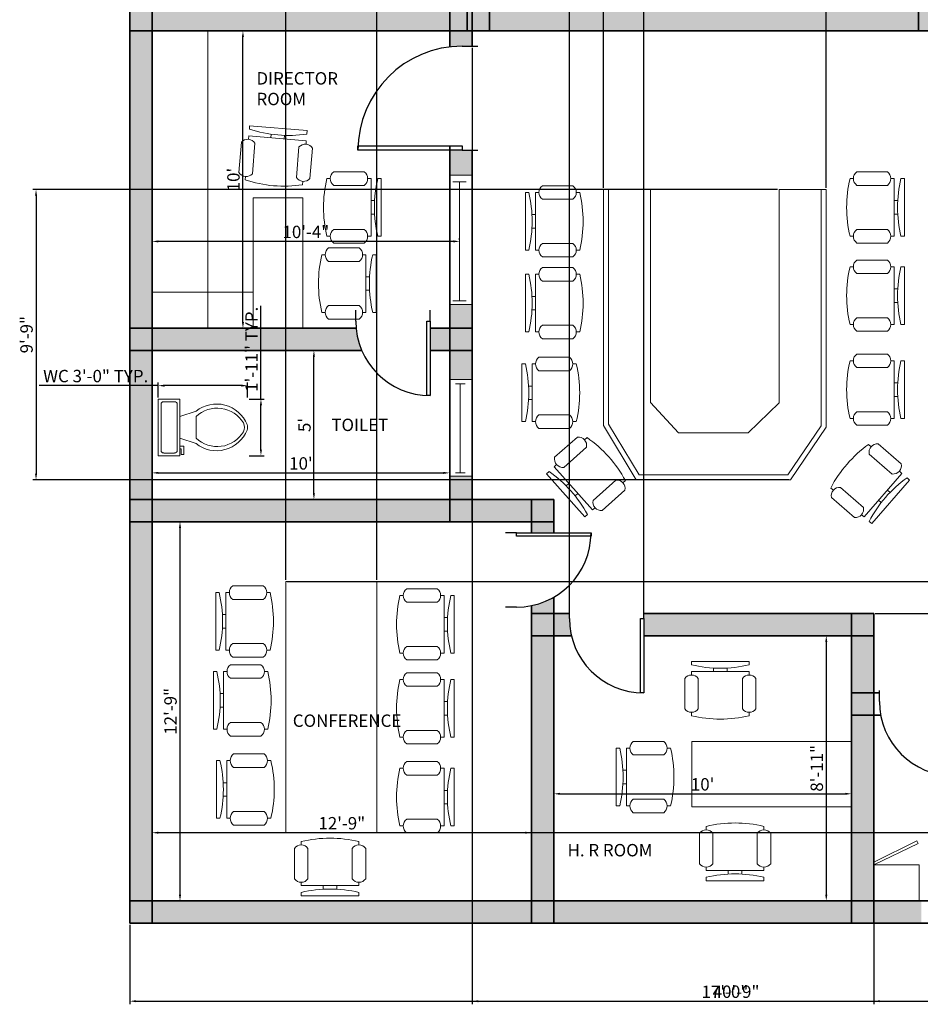
# Model space of a CAD drawing. Units: millimetres. Extents: x 2436 to 3005, y 774 to 1472.
# Tile 1 of 3: x 2436 to 2799, y 774 to 1172. Entities that reach past the tile are written whole.
import ezdxf

# ---------------------------------------------------------------- set-up
doc = ezdxf.new("R2010")
doc.units = ezdxf.units.MM
for name, color, linetype, lineweight in [('A-ANNO-DIMS', 2, 'Continuous', 18), ('A-AREA-IDEN', 10, 'Continuous', 25), ('A-FLOR-CASE', 140, 'Continuous', 18), ('A-FLOR-FIXT', 140, 'Continuous', 18), ('A-WALL-PATT', 3, 'Continuous', 13), ('doors', 30, 'Continuous', 25), ('furniture', 140, 'Continuous', 18), ('walls', 80, 'Continuous', 35), ('window', 190, 'Continuous', 20)]:
    doc.layers.add(name, color=color, linetype=linetype, lineweight=lineweight)
doc.styles.get("Standard").update_dxf_attribs({"font": 'arial.ttf'})
doc.dimstyles.new('ISO-25', dxfattribs={"dimtxt": 5, "dimasz": 2.5, "dimexe": 1.25, "dimexo": 0.625, "dimtad": 1, "dimdec": 0, "dimlunit": 3, "dimtxsty": 'Standard', "dimcen": 2.5, "dimadec": 0, "dimazin": 0, "dimtfac": 1, "dimtdec": 0, "dimtmove": 0, "dimatfit": 3, "dimfxl": 1, "dimarcsym": 0})

# ---------------------------------------------------------------- blocks, each defined once
blk = doc.blocks.new('*U2')
for p, q in [((0, 0), (0, -6)), ((40, 0), (40, -6))]:
    blk.add_line(p, q)
blk.add_lwpolyline([(0, 0), (0, 40), (1.75, 40), (1.75, 0)], close=True)
blk.add_arc((0, 0), 40, 0, 90)
blk = doc.blocks.new('*U4')
for p, q in [((0, 4), (0, 0)), ((36, 4), (36, 0)), ((0, 2), (36, 2))]:
    blk.add_line(p, q)
blk = doc.blocks.new('*U5')
for p, q in [((0, 4), (0, 0)), ((36, 4), (36, 0)), ((0, 2), (36, 2))]:
    blk.add_line(p, q)
blk = doc.blocks.new('Chair - Desk')
for p, q in [((-8.5, 0), (-8.5, -1)), ((-8.5, 0), (8.5, 0)), ((8.5, 0), (8.5, -1)), ((-2, -3), (-2, -1.9355)), ((2, -1.9576), (2, -3)), ((-10.5, -5), (-10.5, -14)), ((-8.5, -3), (-8.5, -4)), ((-8.5, -3), (8.5, -3)), ((-6.5, -14), (-6.5, -5)), ((6.5, -5), (6.5, -14)), ((8.5, -3), (8.5, -4)), ((10.5, -14), (10.5, -5)), ((-8.5, -15), (-8.5, -16)), ((8.5, -15), (8.5, -16))]:
    blk.add_line(p, q)
for centre, radius, start, end in [((0, 34.625), 36.625, 256.5803, 283.4197), ((-8.5, -6.5), 2.5, 36.8699, 143.1301), ((8.5, -6.5), 2.5, 36.8699, 143.1301), ((-8.5, -12.5), 2.5, 216.8699, 323.1301), ((8.5, -12.5), 2.5, 216.8699, 323.1301), ((0, 19.625), 36.625, 256.5803, 283.4197)]:
    blk.add_arc(centre, radius, start, end)
blk = doc.blocks.new('Toilet - top')
for p, q in [((9.5, -6), (9.5, -2)), ((-10, -8.5), (-8, -8.5)), ((-10, -9.5), (-10, -8.5)), ((-7, -9.5), (-10, -9.5)), ((-8, -8.5), (-8, -8)), ((-7, -8), (-7, -9.5)), ((-4, -8), (-6, -14)), ((4, -8), (6, -14)), ((4, -14), (-4, -14))]:
    blk.add_line(p, q)
blk.add_lwpolyline([(10.5, -8), (10.5, 0), (-10.5, 0), (-10.5, -8)], close=True)
for points in [[(-9.5, -2), (-9.5, -6)], [(8.5, -1), (-8.5, -1)], [(-8.5, -7), (8.5, -7)]]:
    blk.add_lwpolyline(points)
for centre, radius, start, end in [((-8.62, -1.88), 0.884, 81.8699, 188.1301), ((8.62, -1.88), 0.884, 351.8699, 98.1301), ((-8.62, -6.12), 0.884, 171.8699, 278.1301), ((8.62, -6.12), 0.884, 261.8699, 8.1301), ((3.52, -21.58), 12.17, 141.4691, 247.9714), ((4.2, -21.82), 11.33, 136.3677, 238.9468), ((-3.52, -21.58), 12.17, 292.0284, 38.5307), ((-4.2, -21.82), 11.33, 301.053, 43.6321), ((0, -27.88), 4, 245.7318, 294.2682), ((0, -29), 4, 254.8605, 285.1395)]:
    blk.add_arc(centre, radius, start, end)
blk = doc.blocks.new('*D17')
at = {"layer": 'A-ANNO-DIMS', "color": 0, "lineweight": -2, "transparency": 16777216}
for p, q in [((2525.92, 1049.62), (2525.92, 1164.62)), ((2526.54, 1167.12), (2527.17, 1167.12)), ((2526.54, 1047.12), (2527.17, 1047.12))]:
    blk.add_line(p, q, dxfattribs=at)
at = {"layer": 'A-ANNO-DIMS', "color": 0, "transparency": 16777216}
for points in [[(2525.5, 1164.62), (2526.33, 1164.62), (2525.92, 1167.12)], [(2525.5, 1049.62), (2526.33, 1049.62), (2525.92, 1047.12)]]:
    blk.add_solid(points, dxfattribs=at)
at = {"layer": 'Defpoints', "color": 0, "transparency": 16777216}
for p in [(2525.92, 1167.12), (2525.92, 1167.12), (2525.92, 1047.12)]:
    blk.add_point(p, dxfattribs=at)
at = {"layer": 'A-ANNO-DIMS', "color": 0, "transparency": 16777216, "insert": (2522.74, 1107.12), "char_height": 5, "attachment_point": 5, "rotation": 90}
blk.add_mtext("10'", dxfattribs=at)
blk = doc.blocks.new('*D18')
at = {"layer": 'A-ANNO-DIMS', "color": 0, "lineweight": -2, "transparency": 16777216}
for p, q in [((2489.3, 1082.81), (2489.3, 1083.44)), ((2610.8, 1082.19), (2491.8, 1082.19)), ((2613.3, 1082.81), (2613.3, 1083.44))]:
    blk.add_line(p, q, dxfattribs=at)
at = {"layer": 'A-ANNO-DIMS', "color": 0, "transparency": 16777216}
for points in [[(2491.8, 1082.6), (2491.8, 1081.77), (2489.3, 1082.19)], [(2610.8, 1082.6), (2610.8, 1081.77), (2613.3, 1082.19)]]:
    blk.add_solid(points, dxfattribs=at)
at = {"layer": 'Defpoints', "color": 0, "transparency": 16777216}
for p in [(2489.3, 1082.19), (2489.3, 1082.19), (2613.3, 1082.19)]:
    blk.add_point(p, dxfattribs=at)
at = {"layer": 'A-ANNO-DIMS', "color": 0, "transparency": 16777216, "insert": (2551.3, 1085.36), "char_height": 5, "attachment_point": 5}
blk.add_mtext('10\'-4"', dxfattribs=at)
blk = doc.blocks.new('*D19')
at = {"layer": 'A-ANNO-DIMS', "color": 0, "lineweight": -2, "transparency": 16777216}
for p, q in [((2553.44, 1038.12), (2555.79, 1038.12)), ((2554.54, 980.62), (2554.54, 1035.62)), ((2553.44, 978.12), (2555.79, 978.12))]:
    blk.add_line(p, q, dxfattribs=at)
at = {"layer": 'A-ANNO-DIMS', "color": 0, "transparency": 16777216}
for points in [[(2554.12, 1035.62), (2554.96, 1035.62), (2554.54, 1038.12)], [(2554.12, 980.62), (2554.96, 980.62), (2554.54, 978.12)]]:
    blk.add_solid(points, dxfattribs=at)
at = {"layer": 'Defpoints', "color": 0, "transparency": 16777216}
for p in [(2552.81, 1038.12), (2554.54, 1038.12), (2552.81, 978.12)]:
    blk.add_point(p, dxfattribs=at)
at = {"layer": 'A-ANNO-DIMS', "color": 0, "transparency": 16777216, "insert": (2551.37, 1008.12), "char_height": 5, "attachment_point": 5, "rotation": 90}
blk.add_mtext("5'", dxfattribs=at)
blk = doc.blocks.new('*D20')
at = {"layer": 'A-ANNO-DIMS', "color": 0, "lineweight": -2, "transparency": 16777216}
for p, q in [((2489.3, 987.7), (2489.3, 990.05)), ((2609.3, 987.7), (2609.3, 990.05)), ((2491.8, 988.8), (2606.8, 988.8))]:
    blk.add_line(p, q, dxfattribs=at)
at = {"layer": 'A-ANNO-DIMS', "color": 0, "transparency": 16777216}
for points in [[(2491.8, 989.22), (2491.8, 988.39), (2489.3, 988.8)], [(2606.8, 989.22), (2606.8, 988.39), (2609.3, 988.8)]]:
    blk.add_solid(points, dxfattribs=at)
at = {"layer": 'Defpoints', "color": 0, "transparency": 16777216}
for p in [(2489.3, 987.08), (2609.3, 988.8), (2609.3, 987.08)]:
    blk.add_point(p, dxfattribs=at)
at = {"layer": 'A-ANNO-DIMS', "color": 0, "transparency": 16777216, "insert": (2549.3, 991.98), "char_height": 5, "attachment_point": 5}
blk.add_mtext("10'", dxfattribs=at)
blk = doc.blocks.new('*D21')
at = {"layer": 'A-ANNO-DIMS', "color": 0, "lineweight": -2, "transparency": 16777216}
for p, q in [((2494.98, 969.12), (2501.78, 969.12)), ((2500.53, 966.62), (2500.53, 818.62)), ((2494.98, 816.12), (2501.78, 816.12))]:
    blk.add_line(p, q, dxfattribs=at)
at = {"layer": 'A-ANNO-DIMS', "color": 0, "transparency": 16777216}
for points in [[(2500.12, 966.62), (2500.95, 966.62), (2500.53, 969.12)], [(2500.12, 818.62), (2500.95, 818.62), (2500.53, 816.12)]]:
    blk.add_solid(points, dxfattribs=at)
at = {"layer": 'Defpoints', "color": 0, "transparency": 16777216}
for p in [(2494.35, 969.12), (2494.35, 816.12), (2500.53, 816.12)]:
    blk.add_point(p, dxfattribs=at)
at = {"layer": 'A-ANNO-DIMS', "color": 0, "transparency": 16777216, "insert": (2497.36, 892.62), "char_height": 5, "attachment_point": 5, "rotation": 90}
blk.add_mtext('12\'-9"', dxfattribs=at)
blk = doc.blocks.new('*D22')
at = {"layer": 'A-ANNO-DIMS', "color": 0, "lineweight": -2, "transparency": 16777216}
for p, q in [((2489.3, 844.27), (2489.3, 844.89)), ((2639.8, 843.64), (2491.8, 843.64)), ((2642.3, 844.27), (2642.3, 844.89))]:
    blk.add_line(p, q, dxfattribs=at)
at = {"layer": 'A-ANNO-DIMS', "color": 0, "transparency": 16777216}
for points in [[(2491.8, 844.06), (2491.8, 843.23), (2489.3, 843.64)], [(2639.8, 844.06), (2639.8, 843.23), (2642.3, 843.64)]]:
    blk.add_solid(points, dxfattribs=at)
at = {"layer": 'Defpoints', "color": 0, "transparency": 16777216}
for p in [(2489.3, 843.64), (2489.3, 843.64), (2642.3, 843.64)]:
    blk.add_point(p, dxfattribs=at)
at = {"layer": 'A-ANNO-DIMS', "color": 0, "transparency": 16777216, "insert": (2565.8, 846.82), "char_height": 5, "attachment_point": 5}
blk.add_mtext('12\'-9"', dxfattribs=at)
blk = doc.blocks.new('*D23')
at = {"layer": 'A-ANNO-DIMS', "color": 0, "lineweight": -2, "transparency": 16777216}
for p, q in [((2651.3, 865.17), (2651.3, 858.09)), ((2771.3, 865.17), (2771.3, 858.09)), ((2653.8, 859.34), (2768.8, 859.34))]:
    blk.add_line(p, q, dxfattribs=at)
at = {"layer": 'A-ANNO-DIMS', "color": 0, "transparency": 16777216}
for points in [[(2653.8, 859.76), (2653.8, 858.92), (2651.3, 859.34)], [(2768.8, 859.76), (2768.8, 858.92), (2771.3, 859.34)]]:
    blk.add_solid(points, dxfattribs=at)
at = {"layer": 'Defpoints', "color": 0, "transparency": 16777216}
for p in [(2651.3, 865.79), (2771.3, 865.79), (2771.3, 859.34)]:
    blk.add_point(p, dxfattribs=at)
at = {"layer": 'A-ANNO-DIMS', "color": 0, "transparency": 16777216, "insert": (2711.3, 862.52), "char_height": 5, "attachment_point": 5}
blk.add_mtext("10'", dxfattribs=at)
blk = doc.blocks.new('*D24')
at = {"layer": 'A-ANNO-DIMS', "color": 0, "lineweight": -2, "transparency": 16777216}
for p, q in [((2758.99, 923.12), (2762.41, 923.12)), ((2761.16, 920.62), (2761.16, 818.62)), ((2761.79, 816.12), (2762.41, 816.12))]:
    blk.add_line(p, q, dxfattribs=at)
at = {"layer": 'A-ANNO-DIMS', "color": 0, "transparency": 16777216}
for points in [[(2760.75, 920.62), (2761.58, 920.62), (2761.16, 923.12)], [(2760.75, 818.62), (2761.58, 818.62), (2761.16, 816.12)]]:
    blk.add_solid(points, dxfattribs=at)
at = {"layer": 'Defpoints', "color": 0, "transparency": 16777216}
for p in [(2758.36, 923.12), (2761.16, 816.12), (2761.16, 816.12)]:
    blk.add_point(p, dxfattribs=at)
at = {"layer": 'A-ANNO-DIMS', "color": 0, "transparency": 16777216, "insert": (2757.99, 869.62), "char_height": 5, "attachment_point": 5, "rotation": 90}
blk.add_mtext('8\'-11"', dxfattribs=at)
blk = doc.blocks.new('*D36')
at = {"layer": 'A-ANNO-DIMS', "color": 0, "lineweight": -2, "transparency": 16777216}
for p, q in [((2491.79, 1019.23), (2491.79, 1025.25)), ((2527.78, 1019.23), (2527.78, 1025.25)), ((2491.79, 1024), (2443.78, 1024)), ((2525.28, 1024), (2494.29, 1024))]:
    blk.add_line(p, q, dxfattribs=at)
at = {"layer": 'A-ANNO-DIMS', "color": 0, "transparency": 16777216}
for points in [[(2494.29, 1024.42), (2494.29, 1023.58), (2491.79, 1024)], [(2525.28, 1024.42), (2525.28, 1023.58), (2527.78, 1024)]]:
    blk.add_solid(points, dxfattribs=at)
at = {"layer": 'Defpoints', "color": 0, "transparency": 16777216}
for p in [(2491.79, 1024), (2491.79, 1018.6), (2527.78, 1018.6)]:
    blk.add_point(p, dxfattribs=at)
at = {"layer": 'A-ANNO-DIMS', "color": 0, "transparency": 16777216, "insert": (2466.54, 1027.21), "char_height": 5, "attachment_point": 5}
blk.add_mtext('WC 3\'-0" TYP.', dxfattribs=at)
blk = doc.blocks.new('*D37')
at = {"layer": 'A-ANNO-DIMS', "color": 0, "lineweight": -2, "transparency": 16777216}
for p, q in [((2533.18, 1018.6), (2533.18, 1056.24)), ((2528.41, 1018.6), (2534.43, 1018.6)), ((2533.18, 998.23), (2533.18, 1016.1)), ((2528.41, 995.73), (2534.43, 995.73))]:
    blk.add_line(p, q, dxfattribs=at)
at = {"layer": 'A-ANNO-DIMS', "color": 0, "transparency": 16777216}
for points in [[(2532.76, 1016.1), (2533.6, 1016.1), (2533.18, 1018.6)], [(2532.76, 998.23), (2533.6, 998.23), (2533.18, 995.73)]]:
    blk.add_solid(points, dxfattribs=at)
at = {"layer": 'Defpoints', "color": 0, "transparency": 16777216}
for p in [(2527.78, 1018.6), (2533.18, 1018.6), (2527.78, 995.73)]:
    blk.add_point(p, dxfattribs=at)
at = {"layer": 'A-ANNO-DIMS', "color": 0, "transparency": 16777216, "insert": (2530.04, 1038.67), "char_height": 5, "attachment_point": 5, "rotation": 90}
blk.add_mtext('1\'-11" TYP.', dxfattribs=at)
blk = doc.blocks.new('*D40')
at = {"layer": 'A-ANNO-DIMS', "color": 0, "lineweight": -2, "transparency": 16777216}
for p, q in [((2480.3, 806.5), (2480.3, 774.42)), ((2969.3, 806.5), (2969.3, 774.42)), ((2482.8, 775.67), (2966.8, 775.67))]:
    blk.add_line(p, q, dxfattribs=at)
at = {"layer": 'A-ANNO-DIMS', "color": 0, "transparency": 16777216}
for points in [[(2482.8, 776.09), (2482.8, 775.26), (2480.3, 775.67)], [(2966.8, 776.09), (2966.8, 775.26), (2969.3, 775.67)]]:
    blk.add_solid(points, dxfattribs=at)
at = {"layer": 'Defpoints', "color": 0, "transparency": 16777216}
for p in [(2480.3, 807.12), (2969.3, 807.12), (2969.3, 775.67)]:
    blk.add_point(p, dxfattribs=at)
at = {"layer": 'A-ANNO-DIMS', "color": 0, "transparency": 16777216, "insert": (2724.8, 778.85), "char_height": 5, "attachment_point": 5}
blk.add_mtext('40\'-9"', dxfattribs=at)
blk = doc.blocks.new('*D42')
at = {"layer": 'A-ANNO-DIMS', "color": 0, "lineweight": -2, "transparency": 16777216}
for p, q in [((2780.3, 931.5), (2780.3, 774.42)), ((2960.3, 890.5), (2960.3, 774.42)), ((2782.8, 775.67), (2957.8, 775.67))]:
    blk.add_line(p, q, dxfattribs=at)
at = {"layer": 'A-ANNO-DIMS', "color": 0, "transparency": 16777216}
for points in [[(2782.8, 776.09), (2782.8, 775.26), (2780.3, 775.67)], [(2957.8, 776.09), (2957.8, 775.26), (2960.3, 775.67)]]:
    blk.add_solid(points, dxfattribs=at)
at = {"layer": 'Defpoints', "color": 0, "transparency": 16777216}
for p in [(2780.3, 932.12), (2960.3, 891.12), (2960.3, 775.67)]:
    blk.add_point(p, dxfattribs=at)
at = {"layer": 'A-ANNO-DIMS', "color": 0, "transparency": 16777216, "insert": (2870.3, 778.85), "char_height": 5, "attachment_point": 5}
blk.add_mtext('15\'-0"', dxfattribs=at)
blk = doc.blocks.new('*D43')
at = {"layer": 'A-ANNO-DIMS', "color": 0, "lineweight": -2, "transparency": 16777216}
for p, q in [((2822.3, 1175.5), (2822.3, 774.42)), ((2618.3, 1160.31), (2618.3, 774.42)), ((2620.8, 775.67), (2819.8, 775.67))]:
    blk.add_line(p, q, dxfattribs=at)
at = {"layer": 'A-ANNO-DIMS', "color": 0, "transparency": 16777216}
for points in [[(2620.8, 776.09), (2620.8, 775.26), (2618.3, 775.67)], [(2819.8, 776.09), (2819.8, 775.26), (2822.3, 775.67)]]:
    blk.add_solid(points, dxfattribs=at)
at = {"layer": 'Defpoints', "color": 0, "transparency": 16777216}
for p in [(2822.3, 1176.12), (2618.3, 1160.93), (2822.3, 775.67)]:
    blk.add_point(p, dxfattribs=at)
at = {"layer": 'A-ANNO-DIMS', "color": 0, "transparency": 16777216, "insert": (2720.3, 778.85), "char_height": 5, "attachment_point": 5}
blk.add_mtext('17\'-0"', dxfattribs=at)
blk = doc.blocks.new('*D44')
at = {"layer": 'A-ANNO-DIMS', "color": 0, "lineweight": -2, "transparency": 16777216}
for p, q in [((2798.92, 1167.12), (3002, 1167.12)), ((3000.75, 1164.62), (3000.75, 934.62)), ((2780.92, 932.12), (3002, 932.12))]:
    blk.add_line(p, q, dxfattribs=at)
at = {"layer": 'A-ANNO-DIMS', "color": 0, "transparency": 16777216}
for points in [[(3000.33, 1164.62), (3001.17, 1164.62), (3000.75, 1167.12)], [(3000.33, 934.62), (3001.17, 934.62), (3000.75, 932.12)]]:
    blk.add_solid(points, dxfattribs=at)
at = {"layer": 'Defpoints', "color": 0, "transparency": 16777216}
for p in [(2798.3, 1167.12), (2780.3, 932.12), (3000.75, 932.12)]:
    blk.add_point(p, dxfattribs=at)
at = {"layer": 'A-ANNO-DIMS', "color": 0, "transparency": 16777216, "insert": (2997.57, 1049.62), "char_height": 5, "attachment_point": 5, "rotation": 90}
blk.add_mtext('19\'-7"', dxfattribs=at)
blk = doc.blocks.new('*D49')
at = {"layer": 'A-ANNO-DIMS', "color": 0, "lineweight": -2, "transparency": 16777216}
for p, q in [((2671.31, 1103.79), (2671.31, 1466.82)), ((2761.12, 1103.79), (2761.12, 1466.82)), ((2673.81, 1465.57), (2758.62, 1465.57))]:
    blk.add_line(p, q, dxfattribs=at)
at = {"layer": 'A-ANNO-DIMS', "color": 0, "transparency": 16777216}
for points in [[(2673.81, 1465.99), (2673.81, 1465.16), (2671.31, 1465.57)], [(2758.62, 1465.99), (2758.62, 1465.16), (2761.12, 1465.57)]]:
    blk.add_solid(points, dxfattribs=at)
at = {"layer": 'Defpoints', "color": 0, "transparency": 16777216}
for p in [(2761.12, 1465.57), (2671.31, 1103.17), (2761.12, 1103.17)]:
    blk.add_point(p, dxfattribs=at)
at = {"layer": 'A-ANNO-DIMS', "color": 0, "transparency": 16777216, "insert": (2716.21, 1468.75), "char_height": 5, "attachment_point": 5}
blk.add_mtext('7\'-6"', dxfattribs=at)
blk = doc.blocks.new('*D50')
at = {"layer": 'A-ANNO-DIMS', "color": 0, "lineweight": -2, "transparency": 16777216}
for p, q in [((2741.49, 1103.17), (2441.22, 1103.17)), ((2442.47, 1100.67), (2442.47, 988.45)), ((2746.13, 985.95), (2441.22, 985.95))]:
    blk.add_line(p, q, dxfattribs=at)
at = {"layer": 'A-ANNO-DIMS', "color": 0, "transparency": 16777216}
for points in [[(2442.06, 1100.67), (2442.89, 1100.67), (2442.47, 1103.17)], [(2442.06, 988.45), (2442.89, 988.45), (2442.47, 985.95)]]:
    blk.add_solid(points, dxfattribs=at)
at = {"layer": 'Defpoints', "color": 0, "transparency": 16777216}
for p in [(2742.12, 1103.17), (2442.47, 985.95), (2746.76, 985.95)]:
    blk.add_point(p, dxfattribs=at)
at = {"layer": 'A-ANNO-DIMS', "color": 0, "transparency": 16777216, "insert": (2439.29, 1044.56), "char_height": 5, "attachment_point": 5, "rotation": 90}
blk.add_mtext('9\'-9"', dxfattribs=at)
blk = doc.blocks.new('*D52')
at = {"layer": 'A-ANNO-DIMS', "color": 0, "lineweight": -2, "transparency": 16777216}
for p, q in [((2657.55, 932.75), (2657.55, 1466.82)), ((2687.55, 932.75), (2687.55, 1466.82)), ((2660.05, 1465.57), (2685.05, 1465.57))]:
    blk.add_line(p, q, dxfattribs=at)
at = {"layer": 'A-ANNO-DIMS', "color": 0, "transparency": 16777216}
for points in [[(2660.05, 1465.99), (2660.05, 1465.16), (2657.55, 1465.57)], [(2685.05, 1465.99), (2685.05, 1465.16), (2687.55, 1465.57)]]:
    blk.add_solid(points, dxfattribs=at)
at = {"layer": 'Defpoints', "color": 0, "transparency": 16777216}
for p in [(2687.55, 1465.57), (2657.55, 932.12), (2687.55, 932.12)]:
    blk.add_point(p, dxfattribs=at)
at = {"layer": 'A-ANNO-DIMS', "color": 0, "transparency": 16777216, "insert": (2672.55, 1468.75), "char_height": 5, "attachment_point": 5}
blk.add_mtext('2\'-6"', dxfattribs=at)
blk = doc.blocks.new('*D53')
at = {"layer": 'A-ANNO-DIMS', "color": 0, "lineweight": -2, "transparency": 16777216}
for p, q in [((2543.16, 945.65), (2543.16, 1466.82)), ((2579.92, 945.65), (2579.92, 1466.82)), ((2545.66, 1465.57), (2577.42, 1465.57))]:
    blk.add_line(p, q, dxfattribs=at)
at = {"layer": 'A-ANNO-DIMS', "color": 0, "transparency": 16777216}
for points in [[(2545.66, 1465.99), (2545.66, 1465.16), (2543.16, 1465.57)], [(2577.42, 1465.99), (2577.42, 1465.16), (2579.92, 1465.57)]]:
    blk.add_solid(points, dxfattribs=at)
at = {"layer": 'Defpoints', "color": 0, "transparency": 16777216}
for p in [(2579.92, 1465.57), (2543.16, 945.02), (2579.92, 945.02)]:
    blk.add_point(p, dxfattribs=at)
at = {"layer": 'A-ANNO-DIMS', "color": 0, "transparency": 16777216, "insert": (2561.54, 1468.75), "char_height": 5, "attachment_point": 5}
blk.add_mtext('3\'-1"', dxfattribs=at)
blk = doc.blocks.new('*D54')
at = {"layer": 'A-ANNO-DIMS', "color": 0, "lineweight": -2, "transparency": 16777216}
for p, q in [((2543.78, 945.02), (3002, 945.02)), ((3000.75, 942.52), (3000.75, 846.17)), ((2543.78, 843.67), (3002, 843.67))]:
    blk.add_line(p, q, dxfattribs=at)
at = {"layer": 'A-ANNO-DIMS', "color": 0, "transparency": 16777216}
for points in [[(3000.33, 942.52), (3001.17, 942.52), (3000.75, 945.02)], [(3000.33, 846.17), (3001.17, 846.17), (3000.75, 843.67)]]:
    blk.add_solid(points, dxfattribs=at)
at = {"layer": 'Defpoints', "color": 0, "transparency": 16777216}
for p in [(2543.16, 945.02), (2543.16, 843.67), (3000.75, 843.67)]:
    blk.add_point(p, dxfattribs=at)
at = {"layer": 'A-ANNO-DIMS', "color": 0, "transparency": 16777216, "insert": (2997.54, 894.35), "char_height": 5, "attachment_point": 5, "rotation": 90}
blk.add_mtext('8\'-5 1/2"', dxfattribs=at)

msp = doc.modelspace()

# ---------------------------------------------------------------- hatches: boundary and pattern name
at = {"layer": 'A-WALL-PATT'}
h = msp.add_hatch(color=256, dxfattribs=at)
h.dxf.hatch_style = 1
h.paths.add_polyline_path([(2822.3, 1374.12), (2489.3, 1374.12), (2489.3, 1365.12), (2822.3, 1365.12)])
h.paths.add_polyline_path([(2831.3, 1374.12), (2822.3, 1374.12), (2822.3, 1365.12), (2831.3, 1365.12)])
h.paths.add_polyline_path([(2831.3, 1365.12), (2822.3, 1365.12), (2822.3, 1353.75), (2824.37, 1353.75, -0.041466), (2831.3, 1353.17)])
h.paths.add_polyline_path([(2960.3, 1425.12), (2951.3, 1425.12), (2951.3, 1305.12), (2960.3, 1305.12)])
h.paths.add_polyline_path([(2960.3, 1434.12), (2951.3, 1434.12), (2951.3, 1425.12), (2960.3, 1425.12)])
h.paths.add_polyline_path([(2951.3, 1434.12), (2831.3, 1434.12), (2831.3, 1425.12), (2951.3, 1425.12)])
h.paths.add_polyline_path([(2831.3, 1434.12), (2822.3, 1434.12), (2822.3, 1425.12), (2831.3, 1425.12)])
h.paths.add_polyline_path([(2489.3, 1374.12), (2480.3, 1374.12), (2480.3, 1365.12), (2489.3, 1365.12)])
h.paths.add_polyline_path([(2489.3, 1365.12), (2480.3, 1365.12), (2480.3, 1354.49), (2489.3, 1354.89)])
h.paths.add_polyline_path([(2489.3, 1313.48, -0.04329), (2482.1, 1312.53), (2480.3, 1312.44), (2480.3, 1176.12), (2489.3, 1176.12)])
h.paths.add_polyline_path([(2489.3, 1176.12), (2480.3, 1176.12), (2480.3, 1167.12), (2489.3, 1167.12)])
h.paths.add_polyline_path([(2609.3, 1176.12), (2489.3, 1176.12), (2489.3, 1167.12), (2609.3, 1167.12)])
h.paths.add_polyline_path([(2625.3, 1176.12), (2618.3, 1176.12), (2618.3, 1167.12), (2625.3, 1167.12)])
h.paths.add_polyline_path([(2618.3, 1176.12), (2616.3, 1176.12), (2616.3, 1167.12), (2618.3, 1167.12)])
h.paths.add_polyline_path([(2616.3, 1176.12), (2609.3, 1176.12), (2609.3, 1167.12), (2616.3, 1167.12)])
h.paths.add_polyline_path([(2618.3, 1167.12), (2609.3, 1167.12), (2609.3, 1160.63, -0.029892), (2614.31, 1160.93), (2618.3, 1160.93)])
h.paths.add_polyline_path([(2625.3, 1305.12), (2616.3, 1305.12), (2616.3, 1176.12), (2618.3, 1176.12), (2625.3, 1176.12)])
h.paths.add_polyline_path([(2798.3, 1176.12), (2625.3, 1176.12), (2625.3, 1167.12), (2798.3, 1167.12)])
h.paths.add_polyline_path([(2807.3, 1176.12), (2798.3, 1176.12), (2798.3, 1167.12), (2807.3, 1167.12)])
h.paths.add_polyline_path([(2831.3, 1176.12), (2822.3, 1176.12), (2822.3, 1167.12), (2831.3, 1167.12)])
h.paths.add_polyline_path([(2822.3, 1176.12), (2807.3, 1176.12), (2807.3, 1167.12), (2822.3, 1167.12)])
h.paths.add_polyline_path([(2951.3, 1176.12), (2831.3, 1176.12), (2831.3, 1167.12), (2951.3, 1167.12)])
h.paths.add_polyline_path([(2960.3, 1176.12), (2951.3, 1176.12), (2951.3, 1167.12), (2960.3, 1167.12)])
h.paths.add_polyline_path([(2960.3, 1296.12), (2951.3, 1296.12), (2951.3, 1176.12), (2960.3, 1176.12)])
h.paths.add_polyline_path([(2960.3, 1305.12), (2951.3, 1305.12), (2951.3, 1296.12), (2960.3, 1296.12)])
h.paths.add_polyline_path([(2951.3, 1305.12), (2831.3, 1305.12), (2831.3, 1296.12), (2951.3, 1296.12)])
h.paths.add_polyline_path([(2822.3, 1305.12), (2807.3, 1305.12), (2807.3, 1296.12), (2822.3, 1296.12)])
h.paths.add_polyline_path([(2831.3, 1305.12), (2822.3, 1305.12), (2822.3, 1296.12), (2831.3, 1296.12)])
h.paths.add_polyline_path([(2831.3, 1311.75), (2824.37, 1311.75), (2822.3, 1311.75), (2822.3, 1305.12), (2831.3, 1305.12)])
h.paths.add_polyline_path([(2807.3, 1305.12), (2798.3, 1305.12), (2798.3, 1296.12), (2807.3, 1296.12)])
h.paths.add_polyline_path([(2807.3, 1236.01), (2798.3, 1236.01), (2798.3, 1221.93), (2801.81, 1221.93, -0.032777), (2807.3, 1221.57)])
h.paths.add_polyline_path([(2831.3, 1167.12), (2822.3, 1167.12), (2822.3, 1139.2), (2826.09, 1139.2, -0.043681), (2831.3, 1138.75)])
h.paths.add_polyline_path([(2807.3, 1179.93), (2801.81, 1179.93), (2798.3, 1179.93), (2798.3, 1176.12), (2807.3, 1176.12)])
h.paths.add_polyline_path([(2927.3, 900.12), (2831.3, 900.12), (2831.3, 891.12), (2927.3, 891.12)])
h.paths.add_polyline_path([(2936.3, 900.12), (2927.3, 900.12), (2927.3, 891.12), (2936.3, 891.12)])
h.paths.add_polyline_path([(2936.3, 905.69), (2927.3, 905.69), (2927.3, 900.12), (2936.3, 900.12)])
h.paths.add_polyline_path([(2831.3, 900.12), (2822.3, 900.12), (2822.3, 891.12), (2831.3, 891.12)])
h.paths.add_polyline_path([(2831.3, 903.84), (2822.3, 903.84), (2822.3, 900.12), (2831.3, 900.12)])
h.paths.add_polyline_path([(2822.3, 900.12), (2812.6, 900.12), (2812.6, 896.54), (2812.6, 891.12), (2822.3, 891.12)])
h.paths.add_polyline_path([(2969.3, 900.12), (2958.95, 900.12), (2936.3, 900.12), (2936.3, 891.12), (2960.3, 891.12), (2960.3, 826.87), (2960.3, 816.12), (2969.3, 816.12), (2969.3, 826.87), (2969.3, 891.12)])
h = msp.add_hatch(color=256, dxfattribs=at)
h.dxf.hatch_style = 1
h.paths.add_polyline_path([(2780.3, 891.12), (2771.3, 891.12), (2771.3, 816.12), (2780.3, 816.12)])
h.paths.add_polyline_path([(2780.3, 900.12), (2771.3, 900.12), (2771.3, 891.12), (2780.3, 891.12)])
h.paths.add_polyline_path([(2780.3, 923.12), (2771.3, 923.12), (2771.3, 900.12), (2780.3, 900.12)])
h.paths.add_polyline_path([(2780.3, 932.12), (2771.3, 932.12), (2771.3, 923.12), (2780.3, 923.12)])
h.paths.add_polyline_path([(2771.3, 932.12), (2687.55, 932.12), (2687.55, 930.04), (2687.55, 923.12), (2771.3, 923.12)])
h.paths.add_polyline_path([(2651.3, 923.12), (2642.3, 923.12), (2642.3, 816.12), (2651.3, 816.12)])
h.paths.add_polyline_path([(2651.3, 816.12), (2642.3, 816.12), (2642.3, 807.12), (2651.3, 807.12)])
h.paths.add_polyline_path([(2771.3, 816.12), (2651.3, 816.12), (2651.3, 807.12), (2771.3, 807.12)])
h.paths.add_polyline_path([(2780.3, 816.12), (2771.3, 816.12), (2771.3, 807.12), (2780.3, 807.12)])
h.paths.add_polyline_path([(2799.5, 816.12), (2780.3, 816.12), (2780.3, 807.12), (2799.5, 807.12)])
h.paths.add_polyline_path([(2960.3, 816.12), (2851.13, 816.12), (2851.13, 807.12), (2960.3, 807.12)])
h.paths.add_polyline_path([(2969.3, 816.12), (2960.3, 816.12), (2960.3, 807.12), (2969.3, 807.12)])
h.paths.add_polyline_path([(2642.3, 816.12), (2489.3, 816.12), (2489.3, 807.12), (2642.3, 807.12)])
h.paths.add_polyline_path([(2489.3, 816.12), (2480.3, 816.12), (2480.3, 807.12), (2489.3, 807.12)])
h.paths.add_polyline_path([(2489.3, 969.12), (2480.3, 969.12), (2480.3, 816.12), (2489.3, 816.12)])
h.paths.add_polyline_path([(2609.3, 978.12), (2489.3, 978.12), (2489.3, 969.12), (2609.3, 969.12)])
h.paths.add_polyline_path([(2489.3, 978.12), (2480.3, 978.12), (2480.3, 969.12), (2489.3, 969.12)])
h.paths.add_polyline_path([(2618.3, 978.12), (2609.3, 978.12), (2609.3, 969.12), (2618.3, 969.12)])
h.paths.add_polyline_path([(2642.3, 978.12), (2618.3, 978.12), (2618.3, 969.12), (2642.3, 969.12)])
h.paths.add_polyline_path([(2651.3, 978.12), (2642.3, 978.12), (2642.3, 969.12), (2651.3, 969.12)])
h.paths.add_polyline_path([(2651.3, 969.12), (2642.3, 969.12), (2642.3, 964.63), (2651.3, 964.63)])
h.paths.add_polyline_path([(2651.3, 932.12), (2642.3, 932.12), (2642.3, 923.12), (2651.3, 923.12)])
h.paths.add_polyline_path([(2657.55, 930.04), (2657.55, 932.12), (2651.3, 932.12), (2651.3, 923.12), (2658.36, 923.12, -0.058212)])
h.paths.add_polyline_path([(2651.3, 938.64, -0.080735), (2642.3, 935.23), (2642.3, 932.12), (2651.3, 932.12)])
h.paths.add_polyline_path([(2489.3, 1038.12), (2480.3, 1038.12), (2480.3, 978.12), (2489.3, 978.12)])
h.paths.add_polyline_path([(2618.3, 987.5), (2609.3, 987.5), (2609.3, 978.12), (2618.3, 978.12)])
h.paths.add_polyline_path([(2618.3, 1038.12), (2609.3, 1038.12), (2609.3, 1026.42), (2618.3, 1026.42)])
h.paths.add_polyline_path([(2489.3, 1047.12), (2480.3, 1047.12), (2480.3, 1038.12), (2489.3, 1038.12)])
h.paths.add_polyline_path([(2618.3, 1047.12), (2609.3, 1047.12), (2609.3, 1038.12), (2618.3, 1038.12)])
h.paths.add_polyline_path([(2489.3, 1167.12), (2480.3, 1167.12), (2480.3, 1047.12), (2489.3, 1047.12)])
h.paths.add_polyline_path([(2618.3, 1118.93), (2614.31, 1118.93), (2609.3, 1118.93), (2609.3, 1108.92), (2618.3, 1108.92)])
h.paths.add_polyline_path([(2618.3, 1056.71), (2609.3, 1056.71), (2609.3, 1047.12), (2618.3, 1047.12)])
edge = h.paths.add_edge_path()
edge.add_arc((2601.4, 1049.98), 30, 185.4674, 203.2834)
edge.add_line((2573.84, 1038.12), (2489.3, 1038.12))
edge.add_line((2489.3, 1038.12), (2489.3, 1047.12))
edge.add_line((2489.3, 1047.12), (2571.54, 1047.12))
h.paths.add_polyline_path([(2601.4, 1047.12), (2601.4, 1038.12), (2609.3, 1038.12), (2609.3, 1047.12)])

# ---------------------------------------------------------------- linework, layer by layer
at = {"layer": 'A-FLOR-CASE'}
for p, q in [((2797.7, 840.35), (2780.3, 831.76)), ((2780.3, 830.65), (2798.2, 839.33)), ((2798.2, 839.33), (2797.7, 840.35)), ((2780.3, 831.76), (2780.3, 830.65))]:
    msp.add_line(p, q, dxfattribs=at)
msp.add_lwpolyline([(2780.3, 816.12), (2798.68, 816.12), (2798.68, 830.65), (2780.3, 830.65)], close=True, dxfattribs=at)
at = {"layer": 'furniture'}
for p, q in [((2671.31, 1007.96), (2671.31, 1103.17)), ((2673.31, 1103.17), (2671.31, 1103.17)), ((2671.31, 1103.17), (2690.31, 1103.17)), ((2673.31, 1068.53), (2673.31, 1103.17)), ((2690.31, 1017.24), (2690.31, 1103.17)), ((2742.12, 1017.04), (2742.12, 1103.17)), ((2742.12, 1103.17), (2761.12, 1103.17)), ((2759.12, 1007.85), (2759.12, 1103.17)), ((2761.12, 1007.24), (2761.12, 1103.17)), ((2673.31, 1008.51), (2673.31, 1068.53)), ((2690.31, 1017.24), (2701.63, 1004.95)), ((2742.12, 1017.04), (2729.62, 1004.95)), ((2684.56, 985.95), (2671.31, 1007.96)), ((2685.69, 987.95), (2673.31, 1008.51)), ((2701.63, 1004.95), (2729.62, 1004.95)), ((2745.69, 987.95), (2759.12, 1007.85)), ((2746.76, 985.95), (2761.12, 1007.24)), ((2684.56, 985.95), (2746.76, 985.95)), ((2685.69, 987.95), (2745.69, 987.95)), ((2685.69, 987.95), (2685.69, 987.95)), ((2745.69, 987.95), (2745.69, 987.95))]:
    msp.add_line(p, q, dxfattribs=at)
for points in [[(2489.3, 1167.12), (2511.75, 1167.12), (2511.75, 1047.12), (2489.3, 1047.12)], [(2530.02, 1047.12), (2550.09, 1047.12), (2550.09, 1099.81), (2530.02, 1099.81)], [(2489.3, 1066.19), (2489.3, 1066.19), (2489.3, 1066.19), (2489.3, 1066.19)], [(2489.3, 1047.12), (2530.02, 1047.12), (2530.02, 1061.69), (2489.3, 1061.69)], [(2489.3, 1060.3), (2489.3, 1060.3), (2489.3, 1060.3), (2489.3, 1060.3)], [(2543.16, 945.02), (2579.92, 945.02), (2579.92, 843.67), (2543.16, 843.67)], [(2771.3, 880.42), (2706.91, 880.42), (2706.91, 854.03), (2771.3, 854.03)]]:
    msp.add_lwpolyline(points, close=True, dxfattribs=at)
at = {"layer": 'walls'}
for p, q in [((2480.3, 1312.44), (2480.3, 807.12)), ((2489.3, 1313.48), (2489.3, 807.12)), ((2616.3, 1305.12), (2616.3, 1167.12)), ((2625.3, 1305.12), (2625.3, 1167.12)), ((2798.3, 1179.93), (2798.3, 1167.12)), ((2609.3, 1176.12), (2609.3, 1160.63)), ((2618.3, 1176.12), (2618.3, 1160.93)), ((2960.3, 1167.12), (2480.3, 1167.12)), ((2609.3, 1120.77), (2609.3, 969.12)), ((2618.3, 1118.93), (2618.3, 969.12)), ((2571.54, 1047.12), (2480.3, 1047.12)), ((2618.3, 1047.12), (2601.4, 1047.12)), ((2573.84, 1038.12), (2480.3, 1038.12)), ((2618.3, 1038.12), (2601.4, 1038.12)), ((2651.3, 978.12), (2480.3, 978.12)), ((2642.3, 978.12), (2642.3, 964.63)), ((2651.3, 978.12), (2651.3, 964.63)), ((2651.3, 969.12), (2480.3, 969.12)), ((2651.3, 938.64), (2651.3, 807.12)), ((2642.3, 935.23), (2642.3, 807.12)), ((2657.55, 932.12), (2642.3, 932.12)), ((2780.3, 932.12), (2687.55, 932.12)), ((2771.3, 932.12), (2771.3, 807.12)), ((2780.3, 932.12), (2780.3, 807.12)), ((2658.36, 923.12), (2642.3, 923.12)), ((2780.3, 923.12), (2687.55, 923.12)), ((2782.6, 900.12), (2771.3, 900.12)), ((2783.09, 891.12), (2771.3, 891.12)), ((2969.3, 816.12), (2480.3, 816.12)), ((2969.3, 807.12), (2480.3, 807.12))]:
    msp.add_line(p, q, dxfattribs=at)
at = {"layer": 'window'}
for p, q in [((2618.3, 1108.92), (2609.3, 1108.92)), ((2618.3, 1056.71), (2609.3, 1056.71)), ((2618.3, 1026.42), (2609.3, 1026.42)), ((2609.3, 987.5), (2618.3, 987.5))]:
    msp.add_line(p, q, dxfattribs=at)

# ---------------------------------------------------------------- block references
at = {"layer": 'A-FLOR-FIXT', "xscale": 1.089104113419681, "yscale": 1.089104113419681, "zscale": 1.089104113419681, "rotation": 90}
msp.add_blockref('Toilet - top', (2491.79, 1007.17), dxfattribs=at)
at = {"layer": 'doors'}
for p, xscale, yscale, zscale, rotation in [((2614.31, 1118.93), 1.05, 1.05, 1.05, 90.00000000000003), ((2601.4, 1049.98), 0.75, 0.75, 0.75, 180), ((2636.3, 964.63), 0.75, 0.75, 0.75, 270), ((2687.55, 930.04), 0.75, 0.75, 0.75, 180), ((2812.6, 896.54), 0.75, 0.75, 0.75, 180)]:
    msp.add_blockref('*U2', p, dxfattribs=dict(at, xscale=xscale, yscale=yscale, zscale=zscale, rotation=rotation))
at = {"layer": 'furniture'}
for p, xscale, yscale, zscale, rotation in [((2540.22, 1127.84), 1.368662376549278, 1.368662376549278, 1.368662376549278, 355.1806042897829), ((2581.68, 1095.9), 1.368662376549279, 1.368662376549279, 1.368662376549279, 270), ((2792.65, 1095.9), 1.368662376549279, 1.368662376549279, 1.368662376549279, 270), ((2639.82, 1090.28), 1.368662376549279, 1.368662376549279, 1.368662376549279, 89.99999999999999), ((2579.65, 1065.19), 1.368662376549279, 1.368662376549279, 1.368662376549279, 270), ((2792.65, 1060.31), 1.368662376549279, 1.368662376549279, 1.368662376549279, 270), ((2639.82, 1057.28), 1.368662376549279, 1.368662376549279, 1.368662376549279, 89.99999999999999), ((2792.65, 1022.39), 1.368662376549279, 1.368662376549279, 1.368662376549279, 270), ((2638.45, 1021.1), 1.368662376549279, 1.368662376549279, 1.368662376549279, 89.99999999999999), ((2656.08, 979.8), 1.368662376549279, 1.368662376549279, 1.368662376549279, 131.7208562822489), ((2787.15, 977.14), 1.368662376549279, 1.368662376549279, 1.368662376549279, 229.0856167799746), ((2514.96, 928.87), 1.368662376549279, 1.368662376549279, 1.368662376549279, 89.99999999999999), ((2611.13, 927.72), 1.368662376549279, 1.368662376549279, 1.368662376549279, 270), ((2514.02, 897.03), 1.368662376549279, 1.368662376549279, 1.368662376549279, 89.99999999999999), ((2611.13, 893.82), 1.368662376549279, 1.368662376549279, 1.368662376549279, 270), ((2676.48, 866.1), 1.368662376549279, 1.368662376549279, 1.368662376549279, 90), ((2515.28, 861.09), 1.368662376549279, 1.368662376549279, 1.368662376549279, 89.99999999999999), ((2611.13, 858), 1.368662376549279, 1.368662376549279, 1.368662376549279, 270), ((2724.38, 824.3), 1.368662376549279, 1.368662376549279, 1.368662376549279, 180.0000000000011), ((2561.05, 818.18), 1.368662376549279, 1.368662376549279, 1.368662376549279, 180.0000000000011)]:
    msp.add_blockref('Chair - Desk', p, dxfattribs=dict(at, xscale=xscale, yscale=yscale, zscale=zscale, rotation=rotation))
at = {"layer": 'furniture', "xscale": 1.368662376549279, "yscale": 1.368662376549279, "zscale": 1.368662376549279}
msp.add_blockref('Chair - Desk', (2718.45, 912.74), dxfattribs=at)
at = {"layer": 'window', "rotation": 90}
for name, p, xscale, yscale, zscale in [('*U4', (2615.96, 1058.19), 1.333333333333333, 1.333333333333333, 1.333333333333333), ('*U5', (2615.57, 988.86), 0.9968650679331311, 0.9968650679331311, 0.9968650679331311)]:
    msp.add_blockref(name, p, dxfattribs=dict(at, xscale=xscale, yscale=yscale, zscale=zscale))

# ---------------------------------------------------------------- texts
at = {"layer": 'A-AREA-IDEN', "char_height": 5, "attachment_point": 1}
for s, width, insert in [('DIRECTOR \\PROOM', 32.2813, (2531.38, 1150.46)), ('TOILET', 41.9742, (2561.58, 1010.67)), ('CONFERENCE', 33.8938, (2546.02, 891.34)), ('H. R ROOM', 40.8613, (2656.83, 839.1))]:
    msp.add_mtext_dynamic_manual_height_columns(s, width=width, gutter_width=12.5, heights=[0], dxfattribs=dict(at, insert=insert))

# ---------------------------------------------------------------- dimensions: what is measured, and where the dimension line sits
at = {"layer": 'A-ANNO-DIMS'}
for base, p1, p2, override, picture, middle in [((2579.92, 1465.57), (2543.16, 945.02), (2579.92, 945.02), {"dimdec": 1, "dimlfac": 1, "dimrnd": 0, "dimzin": 1, "dimdsep": 46, "dimlunit": 4, "dimfrac": 2}, '*D53', (2561.54, 1468.75)), ((2687.55, 1465.57), (2657.55, 932.12), (2687.55, 932.12), {"dimdec": 1, "dimlfac": 1, "dimrnd": 0, "dimzin": 1, "dimdsep": 46, "dimlunit": 4, "dimfrac": 2}, '*D52', (2672.55, 1468.75)), ((2761.12, 1465.57), (2671.31, 1103.17), (2761.12, 1103.17), {"dimdec": 1, "dimlfac": 1, "dimrnd": 0, "dimzin": 1, "dimdsep": 46, "dimlunit": 4, "dimfrac": 2}, '*D49', (2716.21, 1468.75)), ((2822.3, 775.67), (2618.3, 1160.93), (2822.3, 1176.12), {"dimdec": 1, "dimlfac": 1, "dimrnd": 0, "dimzin": 1, "dimdsep": 46, "dimlunit": 4, "dimfrac": 2}, '*D43', (2720.3, 778.85)), ((2489.3, 1082.19), (2613.3, 1082.19), (2489.3, 1082.19), {"dimclrd": 0, "dimclre": 0, "dimclrt": 0}, '*D18', (2551.3, 1085.36)), ((2609.3, 988.8), (2489.3, 987.08), (2609.3, 987.08), {"dimclrd": 0, "dimclre": 0, "dimclrt": 0}, '*D20', (2549.3, 991.98)), ((2960.3, 775.67), (2780.3, 932.12), (2960.3, 891.12), {"dimdec": 1, "dimlfac": 1, "dimrnd": 0, "dimzin": 1, "dimdsep": 46, "dimlunit": 4, "dimfrac": 2}, '*D42', (2870.3, 778.85)), ((2771.3, 859.34), (2651.3, 865.79), (2771.3, 865.79), {"dimclrd": 0, "dimclre": 0, "dimclrt": 0}, '*D23', (2711.3, 862.52)), ((2489.3, 843.64), (2642.3, 843.64), (2489.3, 843.64), {"dimclrd": 0, "dimclre": 0, "dimclrt": 0}, '*D22', (2565.8, 846.82)), ((2969.3, 775.67), (2480.3, 807.12), (2969.3, 807.12), {"dimdec": 1, "dimlfac": 1, "dimrnd": 0, "dimzin": 1, "dimdsep": 46, "dimlunit": 4, "dimfrac": 2}, '*D40', (2724.8, 778.85))]:
    dim = msp.add_linear_dim(base=base, p1=p1, p2=p2, dimstyle='ISO-25', override=override, dxfattribs=at)
    dim.commit()
    dim.dimension.update_dxf_attribs({"geometry": picture, "text_midpoint": middle})
for base, p1, p2, override, picture, middle in [((2525.92, 1167.12), (2525.92, 1047.12), (2525.92, 1167.12), {"dimclrd": 0, "dimclre": 0, "dimclrt": 0}, '*D17', (2522.74, 1107.12)), ((3000.75, 932.12), (2798.3, 1167.12), (2780.3, 932.12), {"dimdec": 1, "dimlfac": 1, "dimrnd": 0, "dimzin": 1, "dimdsep": 46, "dimlunit": 4, "dimfrac": 2}, '*D44', (2997.57, 1049.62)), ((2442.47, 985.95), (2742.12, 1103.17), (2746.76, 985.95), {"dimdec": 1, "dimlfac": 1, "dimrnd": 0, "dimzin": 1, "dimdsep": 46, "dimlunit": 4, "dimfrac": 2}, '*D50', (2439.29, 1044.56)), ((2554.54, 1038.12), (2552.81, 978.12), (2552.81, 1038.12), {"dimclrd": 0, "dimclre": 0, "dimclrt": 0}, '*D19', (2551.37, 1008.12)), ((2500.53, 816.12), (2494.35, 969.12), (2494.35, 816.12), {"dimclrd": 0, "dimclre": 0, "dimclrt": 0}, '*D21', (2497.36, 892.62)), ((3000.7486, 843.6717), (2543.1562, 945.023), (2543.1562, 843.6717), {"dimdec": 1, "dimlfac": 1, "dimrnd": 0, "dimzin": 1, "dimdsep": 46, "dimlunit": 4, "dimfrac": 2}, '*D54', (2997.5383, 894.3473)), ((2761.16, 816.12), (2758.36, 923.12), (2761.16, 816.12), {"dimclrd": 0, "dimclre": 0, "dimclrt": 0}, '*D24', (2757.99, 869.62))]:
    dim = msp.add_linear_dim(base=base, p1=p1, p2=p2, angle=90, dimstyle='ISO-25', override=override, dxfattribs=at)
    dim.commit()
    dim.dimension.update_dxf_attribs({"geometry": picture, "text_midpoint": middle})
for base, p1, p2, angle, text, picture, middle in [((2533.18, 1018.6), (2527.78, 995.73), (2527.78, 1018.6), 90, '<> TYP.', '*D37', (2530.04, 1038.67)), ((2491.79, 1024), (2527.78, 1018.6), (2491.79, 1018.6), 180, 'WC <> TYP.', '*D36', (2466.54, 1027.21))]:
    dim = msp.add_linear_dim(base=base, p1=p1, p2=p2, angle=angle, text=text, dimstyle='ISO-25', override={"dimdec": 1, "dimlfac": 1, "dimrnd": 0, "dimzin": 1, "dimdsep": 46, "dimlunit": 4, "dimfrac": 2}, dxfattribs=at)
    dim.commit()
    dim.dimension.update_dxf_attribs({"geometry": picture, "text_midpoint": middle})

doc.saveas('drawing.dxf')
